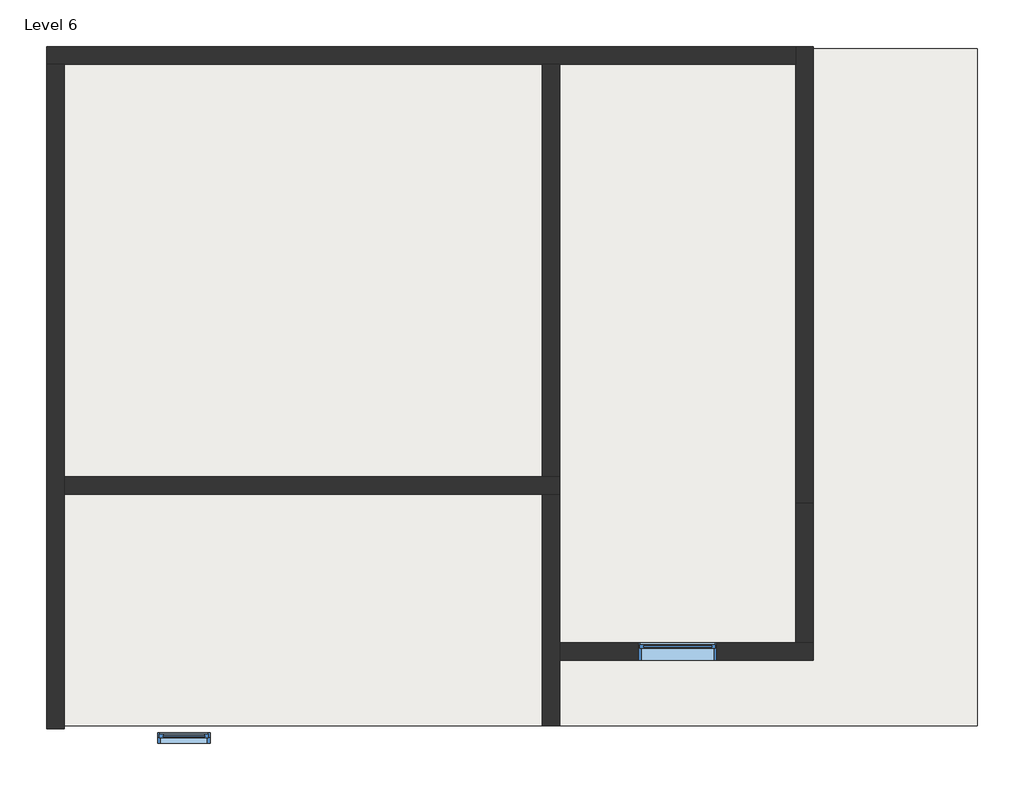
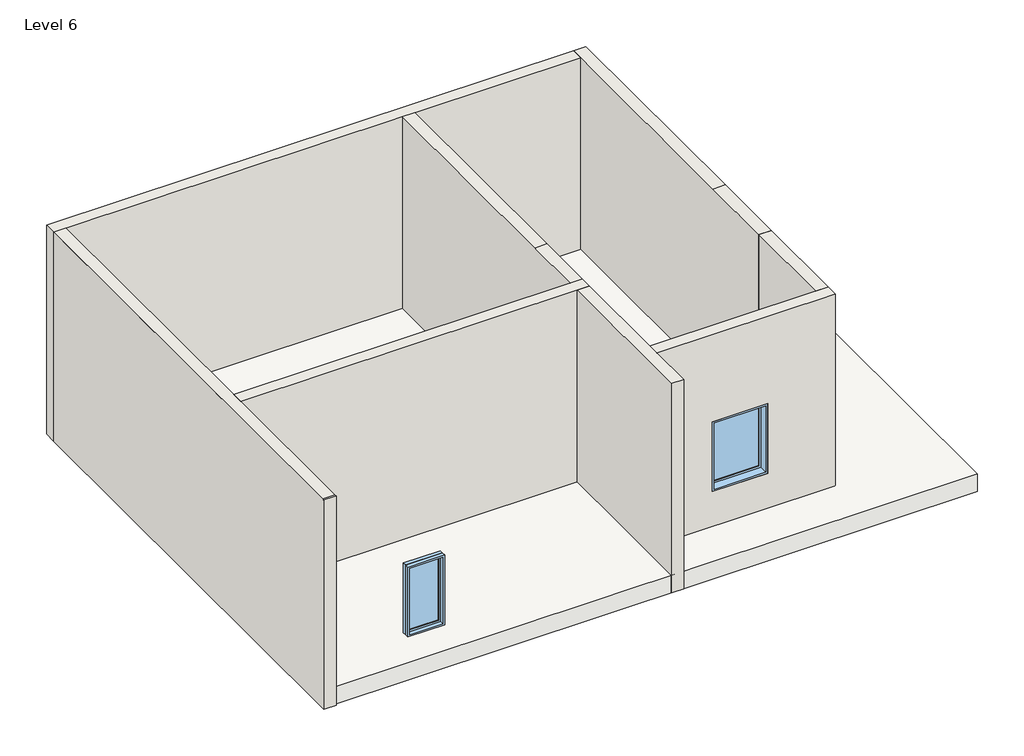
# One storey: 8 walls, 2 windows, 1 roof.
"""IFC4 building model written with IfcOpenShell, lengths in millimetres."""

from ifc_helpers import new_model, si_unit, frame, origin, place, context, project, spatial, polyline, outline, extrude, faceted_brep, transform, mapped, element, save
from components import window_4879aceb, window_e2841890

model = new_model("IFC4")

# Units and contexts
model_context = context("Model", 3, world=origin())
ifc_project = project(units=[si_unit("LENGTHUNIT", "METRE", prefix="MILLI")], contexts=[model_context])

# Site, building, storey
site = spatial("IfcSite", under=ifc_project)
building = spatial("IfcBuilding", under=site)
storey = spatial("IfcBuildingStorey", under=building, Name="Level 6", Elevation=18288.0)

# Roof
placement = place(None, origin())
element("IfcRoof", 1, ObjectType="Generic - 12\"", at=placement, inside=storey, context=model_context, shape_type="SweptSolid", body=[
    extrude(outline(polyline([(-14209.7864811, 10932.8297737), (-3389.3864811, 10932.8297737), (-3389.3864811, 3058.8297737), (-14209.7864811, 3058.8297737), (-14209.7864811, 10932.8297737)])), frame((0.0, 0.0, 18288.0), z_axis=(0.0, 0.0, 1.0), x_axis=(1.0, 0.0, 0.0)), (0.0, 0.0, 1.0), 304.8),
])

# Walls
element("IfcWall", 2, ObjectType="Generic - 8\"", at=placement, inside=storey, context=model_context, shape_type="Brep", body=[
    faceted_brep([(-8246.7304753, 3820.8297737, 18288.0), (-5300.3304753, 3820.8297737, 18288.0), (-5300.3304753, 3820.8297737, 21945.6), (-8246.7304753, 3820.8297737, 21945.6), (-6417.9304753, 3820.8297737, 20421.6), (-6417.9304753, 3820.8297737, 19202.4), (-7332.3304753, 3820.8297737, 19202.4), (-7332.3304753, 3820.8297737, 20421.6), (-8246.7304753, 4024.0297737, 18288.0), (-8246.7304753, 4024.0297737, 21945.6), (-5503.5304753, 4024.0297737, 21945.6), (-5300.3304753, 4024.0297737, 21945.6), (-5300.3304753, 4024.0297737, 18288.0), (-5503.5304753, 4024.0297737, 18288.0), (-6417.9304753, 4024.0297737, 20421.6), (-7332.3304753, 4024.0297737, 20421.6), (-7332.3304753, 4024.0297737, 19202.4), (-6417.9304753, 4024.0297737, 19202.4)], [[[0, 1, 2, 3], [4, 5, 6, 7]], [[8, 9, 10, 11, 12, 13], [14, 15, 16, 17]], [[1, 0, 8, 13, 12]], [[2, 1, 12, 11]], [[0, 3, 9, 8]], [[3, 2, 11, 10, 9]], [[5, 4, 14, 17]], [[6, 5, 17, 16]], [[7, 6, 16, 15]], [[4, 7, 15, 14]]]),
])
element("IfcWall", 3, ObjectType="Generic - 8\"", at=placement, inside=storey, context=model_context, shape_type="SweptSolid", body=[
    extrude(outline(polyline([(-5503.5304753, 4024.0297737), (-5503.5304753, 5650.4732783), (-5300.3304753, 5650.4732783), (-5300.3304753, 4024.0297737), (-5503.5304753, 4024.0297737)])), frame((0.0, 0.0, 18288.0), z_axis=(0.0, 0.0, 1.0), x_axis=(1.0, 0.0, 0.0)), (0.0, 0.0, 1.0), 3657.6),
])
element("IfcWall", 4, ObjectType="Generic - 8\"", at=placement, inside=storey, context=model_context, shape_type="Brep", body=[
    faceted_brep([(-5300.3304753, 5650.4732783, 18288.0), (-5300.3304753, 10958.2297737, 18288.0), (-5300.3304753, 10958.2297737, 21945.6), (-5300.3304753, 6970.4297737, 21945.6), (-5300.3304753, 5650.4732783, 21945.6), (-5503.5304753, 5650.4732783, 18288.0), (-5503.5304753, 5650.4732783, 21945.6), (-5503.5304753, 6970.4297737, 21945.6), (-5503.5304753, 10755.0297737, 21945.6), (-5503.5304753, 10958.2297737, 21945.6), (-5503.5304753, 10958.2297737, 18288.0), (-5503.5304753, 10755.0297737, 18288.0)], [[[0, 1, 2, 3, 4]], [[5, 6, 7, 8, 9, 10, 11]], [[1, 0, 5, 11, 10]], [[0, 4, 6, 5]], [[2, 1, 10, 9]], [[3, 2, 9, 8, 7]], [[4, 3, 7, 6]]]),
])
element("IfcWall", 5, ObjectType="Generic - 8\"", at=placement, inside=storey, context=model_context, shape_type="Brep", body=[
    faceted_brep([(-5503.5304753, 10958.2297737, 18288.0), (-14212.6992777, 10958.2297737, 18288.0), (-14212.6992777, 10958.2297737, 21945.6), (-14209.7864811, 10958.2297737, 21945.6), (-5503.5304753, 10958.2297737, 21945.6), (-5503.5304753, 10755.0297737, 18288.0), (-5503.5304753, 10755.0297737, 21945.6), (-8246.7304753, 10755.0297737, 21945.6), (-8449.9304753, 10755.0297737, 21945.6), (-14009.4992777, 10755.0297737, 21945.6), (-14209.7864811, 10755.0297737, 21945.6), (-14212.6992777, 10755.0297737, 21945.6), (-14212.6992777, 10755.0297737, 18288.0), (-14009.4992777, 10755.0297737, 18288.0), (-8449.9304753, 10755.0297737, 18288.0), (-8246.7304753, 10755.0297737, 18288.0)], [[[0, 1, 2, 3, 4]], [[5, 6, 7, 8, 9, 10, 11, 12, 13, 14, 15]], [[1, 0, 5, 15, 14, 13, 12]], [[0, 4, 6, 5]], [[2, 1, 12, 11]], [[3, 2, 11, 10]], [[4, 3, 10, 9, 8, 7, 6]]]),
])
element("IfcWall", 6, ObjectType="Generic - 8\"", at=placement, inside=storey, context=model_context, shape_type="Brep", body=[
    faceted_brep([(-14212.6992777, 10755.0297737, 18288.0), (-14212.6992777, 3023.9047737, 18288.0), (-14212.6992777, 3023.9047737, 21945.6), (-14212.6992777, 3058.8297737, 21945.6), (-14212.6992777, 10755.0297737, 21945.6), (-14009.4992777, 10755.0297737, 18288.0), (-14009.4992777, 10755.0297737, 21945.6), (-14009.4992777, 5955.2732783, 21945.6), (-14009.4992777, 5752.0732783, 21945.6), (-14009.4992777, 3058.8297737, 21945.6), (-14009.4992777, 3023.9047737, 21945.6), (-14009.4992777, 3023.9047737, 18288.0), (-14009.4992777, 5752.0732783, 18288.0), (-14009.4992777, 5955.2732783, 18288.0), (-14209.7864811, 3023.9047737, 21945.6), (-14209.7864811, 10755.0297737, 21945.6), (-14209.7864811, 3058.8297737, 21945.6)], [[[0, 1, 2, 3, 4]], [[5, 6, 7, 8, 9, 10, 11, 12, 13]], [[1, 0, 5, 13, 12, 11]], [[2, 1, 11, 10, 14]], [[0, 4, 15, 6, 5]], [[4, 3, 16, 15]], [[14, 10, 9, 16]], [[3, 2, 14, 16]], [[16, 9, 8, 7, 6, 15]]]),
])
element("IfcWall", 7, ObjectType="Generic - 8\"", at=placement, inside=storey, context=model_context, shape_type="Brep", body=[
    faceted_brep([(-8246.7304753, 5955.2732783, 18288.0), (-8449.9304753, 5955.2732783, 18288.0), (-14009.4992777, 5955.2732783, 18288.0), (-14009.4992777, 5955.2732783, 21945.6), (-8449.9304753, 5955.2732783, 21945.6), (-8246.7304753, 5955.2732783, 21945.6), (-8246.7304753, 5752.0732783, 18288.0), (-8246.7304753, 5752.0732783, 21945.6), (-8449.9304753, 5752.0732783, 21945.6), (-14009.4992777, 5752.0732783, 21945.6), (-14009.4992777, 5752.0732783, 18288.0), (-8449.9304753, 5752.0732783, 18288.0)], [[[0, 1, 2, 3, 4, 5]], [[6, 7, 8, 9, 10, 11]], [[2, 1, 0, 6, 11, 10]], [[0, 5, 7, 6]], [[3, 2, 10, 9]], [[5, 4, 3, 9, 8, 7]]]),
])
element("IfcWall", 8, ObjectType="Generic - 8\"", at=placement, inside=storey, context=model_context, shape_type="SweptSolid", body=[
    extrude(outline(polyline([(5955.2732783, 18288.0), (5955.2732783, 21945.6), (6970.4297737, 21945.6), (10755.0297737, 21945.6), (10755.0297737, 18288.0), (5955.2732783, 18288.0)])), frame((-8449.9304753, 0.0, 0.0), z_axis=(1.0, 0.0, 0.0), x_axis=(0.0, 1.0, 0.0)), (0.0, 0.0, 1.0), 203.2),
])
element("IfcWall", 9, ObjectType="Generic - 8\"", at=placement, inside=storey, context=model_context, shape_type="Brep", body=[
    faceted_brep([(-8449.9304753, 5752.0732783, 18288.0), (-8449.9304753, 5548.8732783, 18288.0), (-8449.9304753, 3058.8297737, 18288.0), (-8449.9304753, 3058.8297737, 21945.6), (-8449.9304753, 5752.0732783, 21945.6), (-8246.7304753, 5752.0732783, 18288.0), (-8246.7304753, 5752.0732783, 21945.6), (-8246.7304753, 4024.0297737, 21945.6), (-8246.7304753, 3820.8297737, 21945.6), (-8246.7304753, 3058.8297737, 21945.6), (-8246.7304753, 3058.8297737, 18288.0), (-8246.7304753, 3820.8297737, 18288.0), (-8246.7304753, 4024.0297737, 18288.0), (-8246.7304753, 5548.8732783, 18288.0)], [[[0, 1, 2, 3, 4]], [[5, 6, 7, 8, 9, 10, 11, 12, 13]], [[2, 1, 0, 5, 13, 12, 11, 10]], [[3, 2, 10, 9]], [[0, 4, 6, 5]], [[4, 3, 9, 8, 7, 6]]]),
])

# Windows
window_shape = window_4879aceb(model_context)
element("IfcWindow", 10, ObjectType="Fixed : 24\" x 48\"", at=placement, inside=storey, context=model_context, shape_type="MappedRepresentation", body=[
    mapped(window_shape, transform((-12577.4304753, 2919.1297737, 18288.0), x_axis=(1.0, 0.0, 0.0), y_axis=(0.0, 1.0, 0.0), z_axis=(0.0, 0.0, 1.0))),
])
window_2_shape = window_e2841890(model_context)
element("IfcWindow", 11, ObjectType="Fixed : 36\" x 48\"", at=placement, inside=storey, context=model_context, shape_type="MappedRepresentation", body=[
    mapped(window_2_shape, transform((-6837.0304753, 3922.4297737, 18288.0), x_axis=(1.0, 0.0, 0.0), y_axis=(0.0, 1.0, 0.0), z_axis=(0.0, 0.0, 1.0))),
])

save(model, "model.ifc")

# Revit data of these elements
# Type "Generic - 12\""
#   Assembly Code = "B1020"
#   Layers, outside or top first: 1' - 0" no material (function 1)
# Type "Generic - 8\""
#   Assembly Code = "B2010"
#   Layers, outside or top first: 0' - 8" no material (function 1)
# Type "Fixed : 24\" x 48\""
#   Type Mark = "2"
#   Construction Type Id = "GSP4R"
#   Assembly Code = "B2020100"
#   Analytic Construction = "1/8 in Pilkington single glazing"
#   Visual Light Transmittance = 0.9
#   Solar Heat Gain Coefficient = 0.78
#   Heat Transfer Coefficient (U) = 0.6496 BTU/(h·ft²·°F)
#   Height = 4' - 0"
#   Default Sill Height = 3' - 0"
#   Width = 2' - 0"
#   Window Inset = 0' - 0 3/4"
#   Define Thermal Properties by = 1
#   Glass Pane Material = Glass
#   Sash Material = Sash
#   Wall Closure = (empty or 0)
# Type "Fixed : 36\" x 48\""
#   Type Mark = "1"
#   Construction Type Id = "GSP4R"
#   Assembly Code = "B2020100"
#   Analytic Construction = "1/8 in Pilkington single glazing"
#   Visual Light Transmittance = 0.9
#   Solar Heat Gain Coefficient = 0.78
#   Heat Transfer Coefficient (U) = 0.6496 BTU/(h·ft²·°F)
#   Height = 4' - 0"
#   Default Sill Height = 3' - 0"
#   Width = 3' - 0"
#   Window Inset = 0' - 0 3/4"
#   Define Thermal Properties by = 1
#   Glass Pane Material = Glass
#   Sash Material = Sash
#   Wall Closure = (empty or 0)
# Element 1 (IfcRoof, "Generic - 12\"")
#   built-in parameter 1001705 = 61 (stored number, unit not read)
#   built-in parameter 1001710 = 33615
#   Phase Created = New Construction
#   Materials on its faces: "Default Roof"
# Elements 2, 3, 4, 5, 6, 7, 8, 9 (IfcWall, "Generic - 8\"")
#   Top Offset = 0' - 0"
#   Base Offset = 0' - 0"
#   Unconnected Height = 12' - 0"
#   wall height = 12' - 0"
#   Phase Created = New Construction
#   Base Constraint = Level 6
#   Materials on its faces: "Default Wall"
# Element 10 (IfcWindow, "Fixed : 24\" x 48\"")
#   Mark = "7"
#   Phase Created = New Construction
#   Materials on its faces: "Sash", "Glass"
# Element 11 (IfcWindow, "Fixed : 36\" x 48\"")
#   Mark = "2"
#   Phase Created = New Construction
#   Materials on its faces: "Sash", "Glass"
# Materials
#   "Glass": class "Glass", colour RGB 0 128 192, transparency 0.75, Description = "Soda Lime Glass", Cost = 0
#   "Sash": class "Wood", colour RGB 224 178 126, transparency 0
#   "Default Roof": colour RGB 88 101 114, transparency 0
#   "Default Wall": colour RGB 128 128 128, transparency 0
